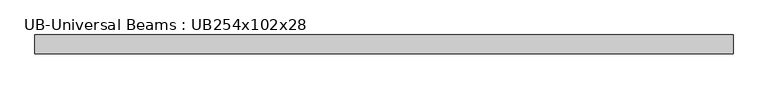
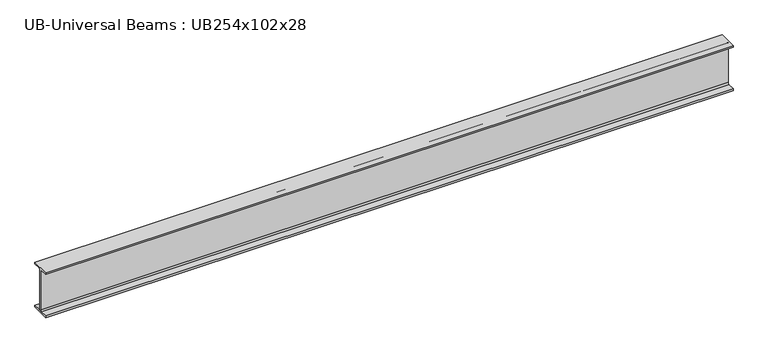
"""IFC4 building model written with IfcOpenShell, lengths in millimetres: beam geometry, UB-Universal Beams : UB254x102x28."""

from ifc_helpers import new_model, si_unit, point, frame, frame_2d, origin, place, context, project, spatial, polyline, circle_curve, trimmed, segment, composite_curve, outline, extrude, source, transform, mapped, element, save


def ub_universal_beams_ub254x102x28_022e5764(model_context):
    return source(origin(), model_context, "Body", "SweptSolid", [
        extrude(outline(composite_curve([segment(polyline([(51.1, -120.2), (51.1, -130.2), (-51.1, -130.2), (-51.1, -120.2), (-10.75, -120.2)]), True, "CONTINUOUS"), segment(trimmed(circle_curve(frame_2d((-10.75, -112.6)), 7.6), [point((-10.75, -120.2))], [point((-3.15, -112.6))], True, "CARTESIAN"), True, "CONTINUOUS"), segment(polyline([(-3.15, -112.6), (-3.15, 112.6)]), True, "CONTINUOUS"), segment(trimmed(circle_curve(frame_2d((-10.75, 112.6)), 7.6), [point((-3.15, 112.6))], [point((-10.75, 120.2))], True, "CARTESIAN"), True, "CONTINUOUS"), segment(polyline([(-10.75, 120.2), (-51.1, 120.2), (-51.1, 130.2), (51.1, 130.2), (51.1, 120.2), (10.75, 120.2)]), True, "CONTINUOUS"), segment(trimmed(circle_curve(frame_2d((10.75, 112.6)), 7.6), [point((10.75, 120.2))], [point((3.15, 112.6))], True, "CARTESIAN"), True, "CONTINUOUS"), segment(polyline([(3.15, 112.6), (3.15, -112.6)]), True, "CONTINUOUS"), segment(trimmed(circle_curve(frame_2d((10.75, -112.6)), 7.6), [point((3.15, -112.6))], [point((10.75, -120.2))], True, "CARTESIAN"), True, "CONTINUOUS"), segment(polyline([(10.75, -120.2), (51.1, -120.2)]), True, "CONTINUOUS")], self_intersect=False)), frame((-1944.65, 0.0, 0.0), z_axis=(1.0, 0.0, 0.0), x_axis=(0.0, 1.0, 0.0)), (0.0, 0.0, 1.0), 3770.3),
    ])


if __name__ == "__main__":
    model = new_model("IFC4")
    model_context = context("Model", 3, world=origin())
    ifc_project = project(units=[si_unit("LENGTHUNIT", "METRE", prefix="MILLI")], contexts=[model_context])
    site = spatial("IfcSite", under=ifc_project)
    building = spatial("IfcBuilding", under=site)
    placement = place(None, origin())
    ub_universal_beams_ub254x102x28_shape = ub_universal_beams_ub254x102x28_022e5764(model_context)
    element("IfcBeam", 1, ObjectType="UB-Universal Beams : UB254x102x28", at=placement, inside=building, context=model_context, shape_type="MappedRepresentation", body=[
        mapped(ub_universal_beams_ub254x102x28_shape, transform((0.0, 0.0, 0.0), x_axis=(1.0, 0.0, 0.0), y_axis=(0.0, 1.0, 0.0), z_axis=(0.0, 0.0, 1.0))),
    ])
    save(model, "model.ifc")

# Revit data of these elements
# Type "UB-Universal Beams : UB254x102x28"
#   Section Name Key = "UB254X102X28"
#   Width = 10.22 cm
#   Web Thickness = 0.63 cm
#   Web Fillet = 0.76 cm
#   Warping Constant = 28000.0 cm⁶
#   Torsional Moment of Inertia = 9.57 cm⁴
#   Section Area = 36.1 cm²
#   Plastic Modulus weak axis = 54.8 cm³
#   Plastic Modulus strong axis = 353.0 cm³
#   Nominal Weight = 28.2999 kgf/m
#   Moment of Inertia weak axis = 179.00 cm⁴
#   Moment of Inertia strong axis = 4005.00 cm⁴
#   Height = 26.04 cm
#   Flange Thickness = 1.0 cm
#   Elastic Modulus weak axis = 34.9 cm³
#   Elastic Modulus strong axis = 308.0 cm³
#   Centroid Vertical = 13.02 cm
#   Centroid Horizontal = 5.11 cm
#   Bolt Spacing = 5.4 cm
#   Length [instance default] = 4' - 11.05512"
#   Structural Material [instance default] = Metal - Steel 43-275
#   Type Comments = ""
#   Assembly Code = ""
# Element 1 (IfcBeam, "UB-Universal Beams : UB254x102x28")
#   Materials on its faces: "Metal - Steel 43-275"
# Materials
#   "Metal - Steel 43-275": class "Metal", colour RGB 247 247 247, transparency 0, Cost = 0
